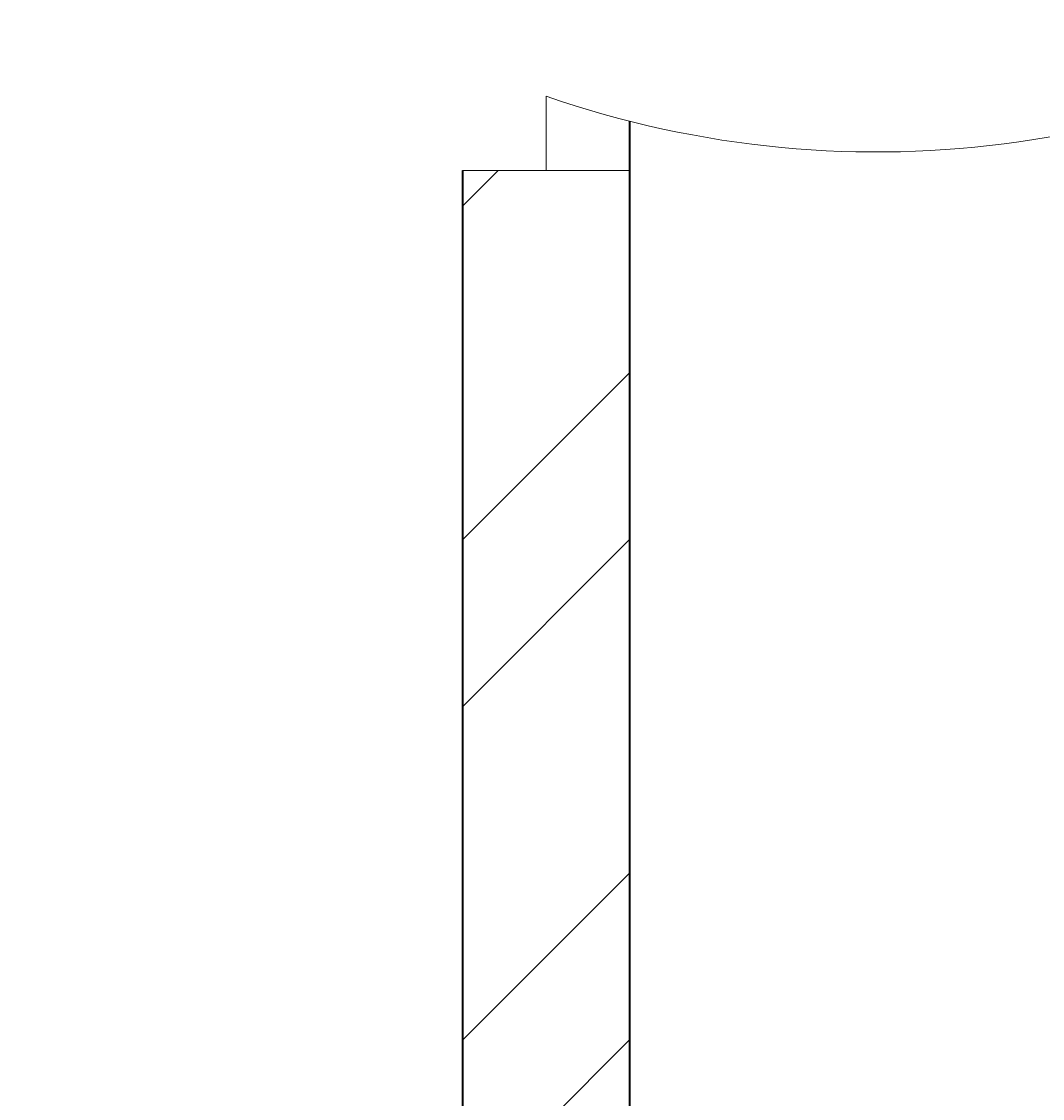
# Model space of a CAD drawing. Units: inches. Extents: x 1962 to 2771, y 1245 to 2660.
# Tile 64 of 114: x 2496 to 2523, y 2062 to 2091. Entities that reach past the tile are written whole.
import ezdxf

# ---------------------------------------------------------------- set-up
doc = ezdxf.new("R2010")
doc.units = ezdxf.units.IN
for name, color, linetype, lineweight in [('A-ANNO-DIMS', 2, 'Continuous', 18), ('A-DOOR', 3, 'Continuous', 18), ('A-WALL', 7, 'Continuous', 35), ('A-WALL-PATT', 252, 'Continuous', 13)]:
    doc.layers.add(name, color=color, linetype=linetype, lineweight=lineweight)
doc.styles.get("Standard").update_dxf_attribs({"font": 'arial.ttf'})
doc.dimstyles.get("Standard").update_dxf_attribs({"dimtxt": 0.18, "dimasz": 0.18, "dimexe": 0.18, "dimexo": 0.0625, "dimgap": 0.09, "dimtad": 0, "dimtih": 1, "dimtoh": 1, "dimdec": 4, "dimzin": 0, "dimdsep": 46, "dimtxsty": 'Standard', "dimcen": 0.09, "dimadec": 0, "dimazin": 0, "dimtfac": 1, "dimtdec": 4, "dimtofl": 0, "dimtmove": 0, "dimatfit": 3, "dimfxl": 1, "dimtolj": 1, "dimtzin": 0, "dimarcsym": 0})

# ---------------------------------------------------------------- blocks, each defined once
blk = doc.blocks.new('*D40')
at = {"layer": 'A-ANNO-DIMS', "color": 0, "lineweight": -2, "transparency": 16777216}
for p, q in [((2072.02, 2033.906), (2072.02, 2583.474)), ((2660.807, 2524.406), (2660.807, 2583.474)), ((2072.2, 2583.294), (2366.02, 2583.294)), ((2660.627, 2583.294), (2366.808, 2583.294))]:
    blk.add_line(p, q, dxfattribs=at)
at = {"layer": 'A-ANNO-DIMS', "color": 0, "transparency": 16777216}
for points in [[(2072.2, 2583.324), (2072.2, 2583.264), (2072.02, 2583.294)], [(2660.627, 2583.324), (2660.627, 2583.264), (2660.807, 2583.294)]]:
    blk.add_solid(points, dxfattribs=at)
at = {"layer": 'Defpoints', "color": 0, "transparency": 16777216}
for p in [(2660.807, 2583.294), (2660.807, 2524.344), (2072.02, 2033.844)]:
    blk.add_point(p, dxfattribs=at)
at = {"layer": 'A-ANNO-DIMS', "color": 0, "transparency": 16777216, "insert": (2366.414, 2583.294), "char_height": 0.18, "attachment_point": 5}
blk.add_mtext('\\A1;588.8', dxfattribs=at)

msp = doc.modelspace()

# ---------------------------------------------------------------- hatches: boundary and pattern name
at = {"layer": 'A-WALL-PATT'}
h = msp.add_hatch(dxfattribs=at)
h.set_pattern_fill('ANSI32', color=256)
h.paths.add_polyline_path([(2090.8074, 2467.3437), (2141.6481, 2467.3437), (2141.6481, 2469.5937), (2141.6481, 2471.8437), (2086.3074, 2471.8437), (2086.3074, 2422.5333), (2090.8074, 2422.5333)])
h.paths.add_polyline_path([(2282.7664, 2471.8437), (2204.8982, 2471.8437), (2204.8982, 2467.3437), (2234.8074, 2467.3437), (2234.8074, 2311.3437), (2228.7492, 2311.3437), (2228.7492, 2306.8437), (2234.8074, 2306.8437), (2331.9227, 2306.8437), (2331.9227, 2309.0937), (2331.9227, 2311.3437), (2239.3074, 2311.3437), (2239.3074, 2467.3437), (2282.7664, 2467.3437), (2282.7664, 2469.5937)])
h.paths.add_polyline_path([(2471.4531, 2519.8437), (2552.011, 2519.8437), (2564.3996, 2519.8437), (2564.3996, 2511.1389), (2568.8996, 2511.1389), (2568.8996, 2524.3437), (2466.9531, 2524.3437), (2466.9531, 2471.8437), (2450.0749, 2471.8437), (2446.4672, 2471.8437), (2446.4672, 2467.3437), (2450.0749, 2467.3437), (2475.9988, 2467.3437), (2475.9988, 2469.5937), (2475.9988, 2471.8437), (2471.4531, 2471.8437)])
h.paths.add_polyline_path([(2575.2231, 2469.5937), (2575.2231, 2471.8437), (2568.8996, 2471.8437), (2568.8996, 2487.1389), (2564.3996, 2487.1389), (2564.3996, 2471.8437), (2556.511, 2471.8437), (2499.2904, 2471.8437), (2499.2904, 2467.3437), (2507.8074, 2467.3437), (2507.8074, 2311.3437), (2414.863, 2311.3437), (2414.863, 2306.8437), (2512.3074, 2306.8437), (2517.0114, 2306.8437), (2517.0114, 2309.0937), (2517.0114, 2311.3437), (2512.3074, 2311.3437), (2512.3074, 2467.3437), (2575.2231, 2467.3437)])
h.paths.add_polyline_path([(2660.8074, 2471.8437), (2600.9602, 2471.8437), (2600.9602, 2467.3437), (2656.3074, 2467.3437), (2656.3074, 2432.5704), (2660.8074, 2432.5704)])
h.paths.add_polyline_path([(2660.8074, 2372.5704), (2656.3074, 2372.5704), (2656.3074, 2311.3437), (2600.276, 2311.3437), (2600.276, 2309.0937), (2600.276, 2306.8437), (2656.3074, 2306.8437), (2656.3074, 2296.2593), (2660.8074, 2296.2593)])
h.paths.add_polyline_path([(2572.3074, 2306.8437), (2577.1385, 2306.8437), (2577.1385, 2311.3437), (2551.082, 2311.3437), (2551.082, 2306.8437), (2567.8074, 2306.8437), (2567.8074, 2258.8437), (2540.0574, 2258.8437), (2540.0574, 2256.5937), (2540.0574, 2254.3437), (2567.8074, 2254.3437), (2656.3074, 2254.3437), (2656.3074, 2236.9085), (2660.8074, 2236.9085), (2660.8074, 2272.2593), (2656.3074, 2272.2593), (2656.3074, 2258.8437), (2572.3074, 2258.8437)])
h.paths.add_polyline_path([(2512.3074, 2254.3437), (2518.8716, 2254.3437), (2518.8716, 2256.5937), (2518.8716, 2258.8437), (2507.8074, 2258.8437), (2507.8074, 2177.8437), (2567.8074, 2177.8437), (2567.8074, 2172.9628), (2572.3074, 2172.9628), (2572.3074, 2177.8437), (2656.3074, 2177.8437), (2656.3074, 2166.4846), (2660.8074, 2166.4846), (2660.8074, 2200.9085), (2656.3074, 2200.9085), (2656.3074, 2182.3437), (2512.3074, 2182.3437)])
h.paths.add_polyline_path([(2656.3074, 2129.8437), (2572.3074, 2129.8437), (2572.3074, 2150.3044), (2570.0574, 2150.3044), (2567.8074, 2150.3044), (2567.8074, 2129.8437), (2507.8074, 2129.8437), (2507.8074, 2116.3027), (2510.0574, 2116.3027), (2512.3074, 2116.3027), (2512.3074, 2125.3437), (2567.8074, 2125.3437), (2572.3074, 2125.3437), (2656.3074, 2125.3437)])
h.paths.add_polyline_path([(2090.8074, 2362.5333), (2086.3074, 2362.5333), (2086.3074, 2298.6242), (2090.8074, 2298.6242), (2090.8074, 2306.8437), (2174.8074, 2306.8437), (2174.8074, 2286.4178), (2179.3074, 2286.4178), (2179.3074, 2306.8437), (2192.8641, 2306.8437), (2192.8641, 2309.0937), (2192.8641, 2311.3437), (2090.8074, 2311.3437)])
h.paths.add_polyline_path([(2209.156, 2258.8437), (2179.3074, 2258.8437), (2179.3074, 2263.2236), (2177.0574, 2263.2236), (2174.8074, 2263.2236), (2174.8074, 2258.8437), (2090.8074, 2258.8437), (2090.8074, 2274.6242), (2086.3074, 2274.6242), (2086.3074, 2238.2967), (2088.5574, 2238.2967), (2090.8074, 2238.2967), (2090.8074, 2254.3437), (2209.156, 2254.3437)])
h.paths.add_polyline_path([(2090.8074, 2177.8437), (2234.8074, 2177.8437), (2234.8074, 2173.1428), (2239.3074, 2173.1428), (2239.3074, 2258.8437), (2230.8442, 2258.8437), (2230.8442, 2256.5937), (2230.8442, 2254.3437), (2234.8074, 2254.3437), (2234.8074, 2182.3437), (2090.8074, 2182.3437), (2090.8074, 2202.2967), (2086.3074, 2202.2967), (2086.3074, 2140.0389), (2090.8074, 2140.0389)])
h.paths.add_polyline_path([(2090.8074, 2080.0389), (2086.3074, 2080.0389), (2086.3074, 2033.8437), (2090.8074, 2033.8437)], flags=17)
h.paths.add_polyline_path([(2244.9405, 2033.8437), (2239.3074, 2033.8437), (2239.3074, 2142.0665), (2237.2592, 2142.0665), (2234.8074, 2142.0665), (2234.8074, 2033.8437), (2090.8074, 2033.8437), (2076.5204, 2033.8437), (2072.0204, 2033.8437), (2072.0204, 2000.4493), (2076.5204, 2000.4493), (2076.5204, 2029.3437), (2090.8074, 2029.3437), (2244.9405, 2029.3437), (2244.9405, 2031.5937)])
h.paths.add_polyline_path([(2234.8074, 1933.3437), (2076.5204, 1933.3437), (2076.5204, 1952.4493), (2074.2704, 1952.4493), (2072.0204, 1952.4493), (2072.0204, 1933.3437), (2072.0204, 1928.8437), (2234.8074, 1928.8437)])
h.paths.add_polyline_path([(2090.8074, 1928.8437), (2086.3074, 1928.8437), (2086.3074, 1906.5013), (2090.8074, 1906.5013)])
h.paths.add_polyline_path([(2090.8074, 1846.5013), (2086.3074, 1846.5013), (2086.3074, 1769.9917), (2088.5574, 1769.9917), (2090.8074, 1769.9917), (2090.8074, 1780.3437), (2234.8074, 1780.3437), (2234.8074, 1708.3437), (2230.3764, 1708.3437), (2230.3764, 1703.8437), (2239.3074, 1703.8437), (2239.3074, 1792.6669), (2237.0574, 1792.6669), (2234.8074, 1792.6669), (2234.8074, 1784.8437), (2090.8074, 1784.8437)])
h.paths.add_polyline_path([(2239.3074, 1928.8437), (2244.9405, 1928.8437), (2244.9405, 1931.0937), (2244.9405, 1933.3437), (2234.8074, 1933.3437), (2234.8074, 1928.8437), (2234.8074, 1825.5949), (2239.3074, 1825.5949)])
h.paths.add_polyline_path([(2148.0425, 1649.0937), (2148.0425, 1651.3437), (2090.8074, 1651.3437), (2090.8074, 1646.8437), (2148.0425, 1646.8437)], flags=0)
h.paths.add_polyline_path([(2207.5601, 1708.3437), (2090.8074, 1708.3437), (2090.8074, 1703.8437), (2174.8074, 1703.8437), (2174.8074, 1651.3437), (2170.4457, 1651.3437), (2170.4457, 1646.8437), (2195.9924, 1646.8437), (2195.9924, 1649.0937), (2195.9924, 1651.3437), (2179.3074, 1651.3437), (2179.3074, 1703.8437), (2207.5601, 1703.8437), (2207.5601, 1706.0937)])
h.paths.add_polyline_path([(2090.8074, 1733.9917), (2086.3074, 1733.9917), (2086.3074, 1696.1032), (2088.5574, 1696.1032), (2090.8074, 1696.1032)])
h.paths.add_polyline_path([(2090.8074, 1672.1032), (2086.3074, 1672.1032), (2086.3074, 1600.3335), (2090.8074, 1600.3335)])
h.paths.add_polyline_path([(2090.8074, 1540.3335), (2086.3074, 1540.3335), (2086.3074, 1486.3437), (2139.6766, 1486.3437), (2139.6766, 1490.8437), (2090.8074, 1490.8437)])
h.paths.add_polyline_path([(2302.3876, 1490.8437), (2239.3074, 1490.8437), (2239.3074, 1646.8437), (2335.9994, 1646.8437), (2335.9994, 1651.3437), (2229.884, 1651.3437), (2229.884, 1646.8437), (2234.8074, 1646.8437), (2234.8074, 1490.8437), (2202.7103, 1490.8437), (2202.7103, 1488.5937), (2202.7103, 1486.3437), (2275.0699, 1486.3437), (2275.0699, 1475.772), (2279.5699, 1475.772), (2279.5699, 1486.3437), (2302.3876, 1486.3437)])
h.paths.add_polyline_path([(2279.5699, 1451.772), (2275.0699, 1451.772), (2275.0699, 1438.3437), (2174.8074, 1438.3437), (2174.8074, 1486.3437), (2179.7922, 1486.3437), (2179.7922, 1490.8437), (2163.3585, 1490.8437), (2163.3585, 1488.5937), (2163.3585, 1486.3437), (2170.3074, 1486.3437), (2170.3074, 1433.8437), (2279.5699, 1433.8437)])
h.paths.add_polyline_path([(2427.2363, 1490.8437), (2375.8074, 1490.8437), (2375.8074, 1646.8437), (2381.6401, 1646.8437), (2381.6401, 1651.3437), (2365.887, 1651.3437), (2365.887, 1649.0937), (2365.887, 1646.8437), (2371.3074, 1646.8437), (2371.3074, 1490.8437), (2327.5627, 1490.8437), (2327.5627, 1488.5937), (2327.5627, 1486.3437), (2371.3074, 1486.3437), (2371.3074, 1433.8437), (2375.8074, 1433.8437), (2375.8074, 1486.3437), (2427.2363, 1486.3437)])
h.paths.add_polyline_path([(2512.3074, 1646.8437), (2519.4351, 1646.8437), (2519.4351, 1649.0937), (2519.4351, 1651.3437), (2507.8074, 1651.3437), (2416.0063, 1651.3437), (2416.0063, 1649.0937), (2416.0063, 1646.8437), (2507.8074, 1646.8437), (2507.8074, 1490.8437), (2497.0532, 1490.8437), (2497.0532, 1488.5937), (2497.0532, 1486.3437), (2574.9344, 1486.3437), (2574.9344, 1476.0181), (2579.4344, 1476.0181), (2579.4344, 1486.3437), (2584.4872, 1486.3437), (2584.3074, 1490.8437), (2512.3074, 1490.8437)])
h.paths.add_polyline_path([(2470.5091, 1486.3437), (2473.9767, 1486.3437), (2473.9767, 1490.8437), (2449.6605, 1490.8437), (2449.6605, 1488.5937), (2449.6605, 1486.3437), (2466.0091, 1486.3437), (2466.0091, 1433.8437), (2470.5091, 1433.8437), (2579.4344, 1433.8437), (2579.4344, 1452.0181), (2574.9344, 1452.0181), (2574.9344, 1438.3437), (2554.5091, 1438.3437), (2470.5091, 1438.3437)])
h.paths.add_polyline_path([(2656.3074, 1490.8437), (2611.86, 1490.8437), (2611.86, 1486.3437), (2656.3074, 1486.3437)])
h.paths.add_polyline_path([(2660.8074, 1532.7007), (2658.5574, 1532.7007), (2656.3074, 1532.7007), (2656.3074, 1486.3437), (2660.8074, 1486.3437)])
h.paths.add_polyline_path([(2660.8074, 1664.9663), (2656.3074, 1664.9663), (2656.3074, 1651.3437), (2602.2313, 1651.3437), (2602.2313, 1646.8437), (2656.3074, 1646.8437), (2656.3074, 1592.7007), (2660.8074, 1592.7007)])
h.paths.add_polyline_path([(2660.8074, 1724.5221), (2656.3074, 1724.5221), (2656.3074, 1703.8437), (2542.4725, 1703.8437), (2542.4725, 1699.3437), (2567.8074, 1699.3437), (2567.8074, 1651.3437), (2552.7766, 1651.3437), (2552.7766, 1649.0937), (2552.7766, 1646.8437), (2577.2878, 1646.8437), (2577.2878, 1649.0937), (2577.2878, 1651.3437), (2572.3074, 1651.3437), (2572.3074, 1699.3437), (2656.3074, 1699.3437), (2656.3074, 1688.9663), (2660.8074, 1688.9663)])
h.paths.add_polyline_path([(2660.8074, 1880.6524), (2656.3074, 1880.6524), (2656.3074, 1832.8437), (2512.3074, 1832.8437), (2512.3074, 1837.8959), (2507.8074, 1837.8959), (2507.8074, 1828.3437), (2567.8074, 1828.3437), (2567.8074, 1804.3437), (2572.3074, 1804.3437), (2572.3074, 1828.3437), (2656.3074, 1828.3437), (2656.3074, 1818.6778), (2660.8074, 1818.6778)])
h.paths.add_polyline_path([(2660.8074, 1794.6778), (2656.3074, 1794.6778), (2656.3074, 1780.3437), (2572.3074, 1780.3437), (2572.3074, 1783.0303), (2570.0574, 1783.0303), (2567.8074, 1783.0303), (2567.8074, 1780.3437), (2507.8074, 1780.3437), (2507.8074, 1699.3437), (2517.8858, 1699.3437), (2517.8858, 1701.5937), (2517.8858, 1703.8437), (2512.3074, 1703.8437), (2512.3074, 1775.8437), (2656.3074, 1775.8437), (2656.3074, 1760.5221), (2660.8074, 1760.5221)])
h.paths.add_polyline_path([(2660.8074, 1981.3437), (2660.8074, 2020.2808), (2658.5574, 2020.2808), (2656.3074, 2020.2808), (2656.3074, 1981.3437), (2512.3074, 1981.3437), (2512.3074, 2086.6996), (2507.8074, 2086.6996), (2507.8074, 1981.3437), (2375.8074, 1981.3437), (2375.8074, 1986.8505), (2373.5574, 1986.8505), (2371.3074, 1986.8505), (2371.3074, 1973.2607), (2375.8074, 1973.2607), (2375.8074, 1976.8437), (2507.8074, 1976.8437), (2507.8074, 1865.4281), (2510.0574, 1865.4281), (2512.3074, 1865.4281), (2512.3074, 1976.8437), (2660.8074, 1976.8437)])
h.paths.add_polyline_path([(2375.8074, 1940.297), (2373.5574, 1940.297), (2371.3074, 1940.297), (2371.3074, 1933.3437), (2278.4434, 1933.3437), (2278.4434, 1928.8437), (2371.3074, 1928.8437), (2371.3074, 1651.3437), (2375.8074, 1651.3437)])
h.paths.add_polyline_path([(2660.8074, 1976.8437), (2656.3074, 1976.8437), (2656.3074, 1940.6524), (2660.8074, 1940.6524)], flags=17)
h.paths.add_polyline_path([(2660.8074, 2142.4846), (2656.3074, 2142.4846), (2656.3074, 2080.2808), (2660.8074, 2080.2808)])
h.paths.add_polyline_path([(2381.4189, 2311.3437), (2375.8074, 2311.3437), (2375.8074, 2467.3437), (2424.7242, 2467.3437), (2424.7242, 2469.5937), (2424.7242, 2471.8437), (2375.8074, 2471.8437), (2375.8074, 2524.3437), (2371.3074, 2524.3437), (2371.3074, 2471.8437), (2307.2097, 2471.8437), (2307.2097, 2467.3437), (2371.3074, 2467.3437), (2371.3074, 2311.3437), (2366.8901, 2311.3437), (2366.8901, 2306.8437), (2371.3074, 2306.8437), (2371.3074, 2033.8437), (2279.6589, 2033.8437), (2279.6589, 2029.3437), (2371.3074, 2029.3437), (2371.3074, 2014.2598), (2375.8074, 2014.2598), (2375.8074, 2306.8437), (2381.4189, 2306.8437)])
h.paths.add_polyline_path([(2263.3074, 2524.3437), (2170.3074, 2524.3437), (2170.3074, 2519.8437), (2170.3074, 2471.8437), (2165.0312, 2471.8437), (2165.0312, 2467.3437), (2179.6721, 2467.3437), (2179.6721, 2469.5161), (2179.6721, 2471.8437), (2174.8074, 2471.8437), (2174.8074, 2519.8437), (2258.8074, 2519.8437), (2258.8074, 2511.6436), (2263.3074, 2511.6436)])
h.paths.add_polyline_path([(2245.0232, 1361.4123), (2492.9468, 1361.4123), (2492.9468, 1398.505), (2245.0232, 1398.505)], flags=9)
h.paths.add_polyline_path([(2388.1434, 2086.6936), (2425.0704, 2086.6936), (2425.0704, 2105.3509), (2388.1434, 2105.3509)], flags=9)
h.paths.add_polyline_path([(2404.922, 2242.6744), (2445.7337, 2242.6744), (2445.7337, 2261.3318), (2404.922, 2261.3318)], flags=9)
h.paths.add_polyline_path([(2269.4107, 2156.7935), (2306.3378, 2156.7935), (2306.3378, 2175.4508), (2269.4107, 2175.4508)], flags=9)
h.paths.add_polyline_path([(2269.3277, 2233.4343), (2306.2547, 2233.4343), (2306.2547, 2252.0917), (2269.3277, 2252.0917)], flags=9)
h.paths.add_polyline_path([(2431.6052, 2320.6922), (2470.4456, 2320.6922), (2470.4456, 2339.3495), (2431.6052, 2339.3495)], flags=25)
h.paths.add_polyline_path([(2249.6902, 2315.7608), (2288.5306, 2315.7608), (2288.5306, 2334.4182), (2249.6902, 2334.4182)], flags=25)
h.paths.add_polyline_path([(2096.9301, 2314.3181), (2135.7704, 2314.3181), (2135.7704, 2332.9755), (2096.9301, 2332.9755)], flags=25)
h.paths.add_polyline_path([(2134.3475, 2285.7089), (2161.4655, 2285.7089), (2161.4655, 2304.3662), (2134.3475, 2304.3662)], flags=9)
h.paths.add_polyline_path([(2126.5155, 2209.4076), (2159.9227, 2209.4076), (2159.9227, 2228.065), (2126.5155, 2228.065)], flags=25)
h.paths.add_polyline_path([(2110.5753, 2141.5299), (2149.4157, 2141.5299), (2149.4157, 2160.1872), (2110.5753, 2160.1872)], flags=25)
h.paths.add_polyline_path([(2249.8618, 1968.3317), (2286.3966, 1968.3317), (2286.3966, 1986.989), (2249.8618, 1986.989)], flags=9)
h.paths.add_polyline_path([(2395.9507, 1777.0051), (2436.7624, 1777.0051), (2436.7624, 1795.6625), (2395.9507, 1795.6625)], flags=9)
h.paths.add_polyline_path([(2398.5259, 1888.5651), (2435.0062, 1888.5651), (2435.0062, 1907.2224), (2398.5259, 1907.2224)], flags=25)
h.paths.add_polyline_path([(2259.3506, 1728.3559), (2296.2776, 1728.3559), (2296.2776, 1747.0132), (2259.3506, 1747.0132)], flags=9)
h.paths.add_polyline_path([(2271.3698, 1845.268), (2308.2968, 1845.268), (2308.2968, 1863.9253), (2271.3698, 1863.9253)], flags=9)
h.paths.add_polyline_path([(2120.9355, 1786.3027), (2159.7759, 1786.3027), (2159.7759, 1804.9601), (2120.9355, 1804.9601)], flags=25)
h.paths.add_polyline_path([(2121.3164, 1732.1043), (2154.7236, 1732.1043), (2154.7236, 1750.7616), (2121.3164, 1750.7616)], flags=25)
h.paths.add_polyline_path([(2118.3706, 1678.8997), (2147.5282, 1678.8997), (2147.5282, 1697.557), (2118.3706, 1697.557)], flags=25)
h.paths.add_polyline_path([(2385.9227, 1493.557), (2424.763, 1493.557), (2424.763, 1512.2143), (2385.9227, 1512.2143)], flags=25)
h.paths.add_polyline_path([(2248.7058, 1500.0256), (2287.5462, 1500.0256), (2287.5462, 1518.6829), (2248.7058, 1518.6829)], flags=25)
h.paths.add_polyline_path([(2104.1669, 1617.3771), (2143.0073, 1617.3771), (2143.0073, 1636.0344), (2104.1669, 1636.0344)], flags=9)
h.paths.add_polyline_path([(2096.0714, 1447.8824), (2137.3845, 1447.8824), (2137.3845, 1458.1859), (2096.0714, 1458.1859)], flags=9)
h.paths.add_polyline_path([(2180.6114, 1440.325), (2209.7689, 1440.325), (2209.7689, 1458.9823), (2180.6114, 1458.9823)], flags=25)
h.paths.add_polyline_path([(2316.1698, 1447.9637), (2357.4829, 1447.9637), (2357.4829, 1458.2673), (2316.1698, 1458.2673)], flags=9)
h.paths.add_polyline_path([(2397.6187, 1447.9637), (2438.9318, 1447.9637), (2438.9318, 1458.2673), (2397.6187, 1458.2673)], flags=9)
h.paths.add_polyline_path([(2473.0778, 1439.5953), (2502.2354, 1439.5953), (2502.2354, 1458.2527), (2473.0778, 1458.2527)], flags=25)
h.paths.add_polyline_path([(2589.7027, 1447.8819), (2631.0158, 1447.8819), (2631.0158, 1458.1855), (2589.7027, 1458.1855)], flags=9)
h.paths.add_polyline_path([(2522.4009, 1497.5285), (2561.2413, 1497.5285), (2561.2413, 1516.1859), (2522.4009, 1516.1859)], flags=25)
h.paths.add_polyline_path([(2579.6565, 1671.3482), (2608.8141, 1671.3482), (2608.8141, 1690.0056), (2579.6565, 1690.0056)], flags=25)
h.paths.add_polyline_path([(2544.7038, 1725.5064), (2578.1111, 1725.5064), (2578.1111, 1744.1637), (2544.7038, 1744.1637)], flags=25)
h.paths.add_polyline_path([(2578.1191, 1807.472), (2607.2766, 1807.472), (2607.2766, 1826.1293), (2578.1191, 1826.1293)], flags=25)
h.paths.add_polyline_path([(2595.0614, 1835.1839), (2633.9018, 1835.1839), (2633.9018, 1853.8413), (2595.0614, 1853.8413)], flags=25)
h.paths.add_polyline_path([(2567.0097, 2097.7035), (2605.8501, 2097.7035), (2605.8501, 2116.3609), (2567.0097, 2116.3609)], flags=9)
h.paths.add_polyline_path([(2586.644, 2134.6454), (2615.8015, 2134.6454), (2615.8015, 2153.3027), (2586.644, 2153.3027)], flags=9)
h.paths.add_polyline_path([(2544.6185, 2212.6783), (2578.0258, 2212.6783), (2578.0258, 2231.3356), (2544.6185, 2231.3356)], flags=25)
h.paths.add_polyline_path([(2577.0273, 2256.9023), (2606.1849, 2256.9023), (2606.1849, 2275.5597), (2577.0273, 2275.5597)], flags=24)
h.paths.add_polyline_path([(2605.2683, 2315.2821), (2644.1087, 2315.2821), (2644.1087, 2333.9395), (2605.2683, 2333.9395)], flags=25)
h.paths.add_polyline_path([(2583.1244, 2496.1815), (2624.4375, 2496.1815), (2624.4375, 2506.4851), (2583.1244, 2506.4851)], flags=9)
h.paths.add_polyline_path([(2474.761, 2497.0823), (2503.9185, 2497.0823), (2503.9185, 2515.7397), (2474.761, 2515.7397)], flags=25)
h.paths.add_polyline_path([(2387.5787, 2494.2563), (2428.902, 2494.2563), (2428.902, 2504.5598), (2387.5787, 2504.5598)], flags=9)
h.paths.add_polyline_path([(2300.1657, 2500.1564), (2341.4788, 2500.1564), (2341.4788, 2510.46), (2300.1657, 2510.46)], flags=25)
h.paths.add_polyline_path([(2176.8589, 2497.5843), (2206.0165, 2497.5843), (2206.0165, 2516.2416), (2176.8589, 2516.2416)], flags=25)
h.paths.add_polyline_path([(2097.4668, 2494.9762), (2138.7799, 2494.9762), (2138.7799, 2505.2798), (2097.4668, 2505.2798)], flags=9)

# ---------------------------------------------------------------- linework, layer by layer
at = {"layer": 'A-DOOR'}
for p, q in [((2510.0574, 2086.6996), (2510.0574, 2088.6996)), ((2512.3074, 2086.6996), (2507.8074, 2086.6996)), ((2507.8074, 2086.6996), (2510.0574, 2086.6996))]:
    msp.add_line(p, q, dxfattribs=at)
msp.add_arc((2518.9529, 2114.3027), 27.1044, 250.84069, 360, dxfattribs=at)
at = {"layer": 'A-WALL'}
for p, q in [((2512.3074, 2088.0256), (2512.3074, 1981.3437)), ((2507.8074, 2086.6996), (2507.8074, 1981.3437)), ((2507.8074, 2086.6996), (2507.8074, 1981.3437))]:
    msp.add_line(p, q, dxfattribs=at)

# ---------------------------------------------------------------- dimensions: what is measured, and where the dimension line sits
at = {"layer": 'A-ANNO-DIMS'}
dim = msp.add_linear_dim(base=(2660.8074, 2583.2937), p1=(2072.0204, 2033.8437), p2=(2660.8074, 2524.3437), dimstyle='Standard', override={"dimdec": 1, "dimlfac": 1, "dimrnd": 0, "dimzin": 0, "dimdsep": 46, "dimlunit": 2}, dxfattribs=at)
dim.commit()
dim.dimension.update_dxf_attribs({"geometry": '*D40', "text_midpoint": (2366.4139, 2583.2937)})

doc.saveas('drawing.dxf')
